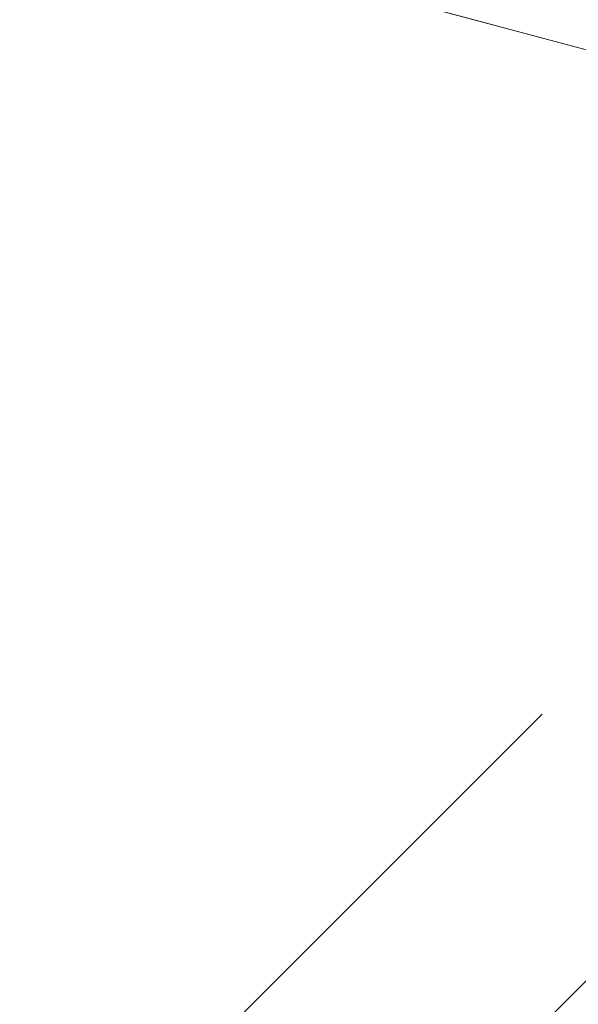
# Model space of a CAD drawing. Units: inches. Extents: x 375 to 1122, y 27 to 1069.
# Tile 132 of 155: x 723.463 to 725.559, y 900.211 to 903.908. Entities that reach past the tile are written whole.
import ezdxf

# ---------------------------------------------------------------- set-up
doc = ezdxf.new("R2010")
doc.units = ezdxf.units.IN
doc.layers.add('A-ANNO-DIMS', color=2, linetype='Continuous', lineweight=18)
doc.layers.add('Furniture', color=30, linetype='Continuous', lineweight=18)
doc.styles.get("Standard").update_dxf_attribs({"font": 'arial.ttf'})
doc.dimstyles.new('ISO-25', dxfattribs={"dimtxt": 12, "dimasz": 2.5, "dimexe": 1.5, "dimexo": 1.5, "dimtad": 1, "dimdec": 1, "dimlunit": 3, "dimtxsty": 'Standard', "dimblk": 'ARCHTICK', "dimcen": 2.5, "dimadec": 0, "dimazin": 0, "dimtfac": 1, "dimtdec": 1, "dimtmove": 0, "dimatfit": 3, "dimfxl": 1.5, "dimfxlon": 1, "dimarcsym": 0})

# ---------------------------------------------------------------- blocks, each defined once
blk = doc.blocks.new('A$C403C54AD')
for p, q in [((0.906853, 1.059765, -0.000599), (1.019435, 0.947232, -0.000599)), ((0.925555, 1.011934, -0.000599), (1.038137, 0.8994, -0.000599))]:
    blk.add_line(p, q)
at = {"linetype": 'ByBlock', "invisible_edges": 5}
for points in [[(0.818605, 0.976049, -0.033549), (0.847931, 0.959118, -0.024314), (0.86649, 1.028382, -0.024314), (0.832628, 1.028382, -0.033549)], [(0.847931, 0.959118, -0.019696), (0.831935, 0.968354, -0.019696), (0.84802, 1.028382, -0.019696), (0.86649, 1.028382, -0.019696)]]:
    blk.add_3dface(points, dxfattribs=at)
at = {"linetype": 'ByBlock'}
blk.add_3dface([(0.847931, 0.959118, -0.024314), (0.847931, 0.959118, -0.019696), (0.86649, 1.028382, -0.019696), (0.86649, 1.028382, -0.024314)], dxfattribs=at)
blk = doc.blocks.new('_ArchTick')
at = {"color": 0, "linetype": 'ByBlock', "const_width": 0.15}
blk.add_lwpolyline([(-0.5, -0.5), (0.5, 0.5)], dxfattribs=at)
blk = doc.blocks.new('*D73')
at = {"layer": 'A-ANNO-DIMS', "color": 0, "lineweight": -2, "transparency": 16777216}
for p, q in [((686.7573, 932.4277), (686.7573, 929.4277)), ((770.7573, 932.4277), (770.7573, 929.4277)), ((686.7573, 930.9277), (770.7573, 930.9277)), ((770.7573, 930.9277), (987.6096, 930.9277))]:
    blk.add_line(p, q, dxfattribs=at)
at = {"layer": 'Defpoints', "color": 0, "transparency": 16777216}
for p in [(686.7573, 943.5277), (770.7573, 943.5277), (770.7573, 930.9277)]:
    blk.add_point(p, dxfattribs=at)
at = {"layer": 'A-ANNO-DIMS', "color": 0, "lineweight": -2, "transparency": 16777216, "xscale": 2.5, "yscale": 2.5, "zscale": 2.5, "rotation": 180}
blk.add_blockref('_ArchTick', (686.7573, 930.9277), dxfattribs=at)
at = {"layer": 'A-ANNO-DIMS', "color": 0, "lineweight": -2, "transparency": 16777216, "xscale": 2.5, "yscale": 2.5, "zscale": 2.5}
blk.add_blockref('_ArchTick', (770.7573, 930.9277), dxfattribs=at)
at = {"layer": 'A-ANNO-DIMS', "color": 0, "transparency": 16777216, "insert": (880.4335, 937.7573), "char_height": 12, "attachment_point": 5}
blk.add_mtext('2-PANEL SLIDER 7\'-0" TYP.', dxfattribs=at)

msp = doc.modelspace()

# ---------------------------------------------------------------- block references
at = {"layer": 'Furniture', "xscale": 39.9918517141215, "yscale": 39.9918517141215, "zscale": 39.9918517141215, "rotation": 270}
msp.add_blockref('A$C403C54AD', (684.9549, 938.3156, 0.024), dxfattribs=at)

# ---------------------------------------------------------------- dimensions: what is measured, and where the dimension line sits
at = {"layer": 'A-ANNO-DIMS'}
dim = msp.add_linear_dim(base=(770.7573, 930.9277), p1=(686.7573, 943.5277), p2=(770.7573, 943.5277), text='2-PANEL SLIDER <> TYP.', dimstyle='ISO-25', override={"dimdec": 1, "dimlfac": 1, "dimrnd": 0, "dimzin": 1, "dimdsep": 46, "dimlunit": 4, "dimfrac": 2}, dxfattribs=at)
dim.commit()
dim.dimension.update_dxf_attribs({"geometry": '*D73', "text_midpoint": (880.4335, 937.7573)})

doc.saveas('drawing.dxf')
